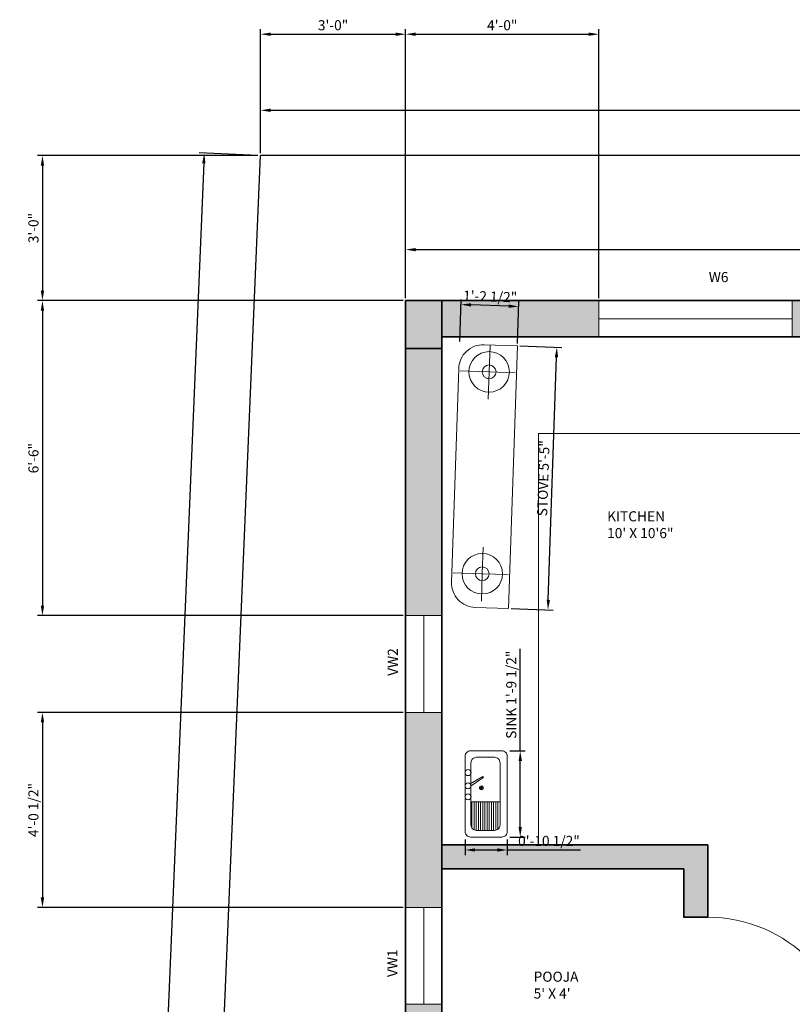
# Model space of a CAD drawing. Units: inches. Extents: x 5395 to 6469, y -203 to 448.
# Tile 3 of 7: x 5395 to 5587, y 204 to 448. Entities that reach past the tile are written whole.
import ezdxf

# ---------------------------------------------------------------- set-up
doc = ezdxf.new("R2010")
doc.units = ezdxf.units.IN
for name, color, linetype, lineweight in [('A-ANNO-DIMS', 2, 'Continuous', 18), ('A-ANNO-TEXT', 6, 'Continuous', 18), ('A-AREA-IDEN', 6, 'Continuous', 18), ('A-COLS', 7, 'Continuous', 35), ('A-COLS-PATT', 2, 'Continuous', 13), ('A-EQPM', 70, 'Continuous', 18), ('A-FLOR-CASE', 32, 'Continuous', 18), ('A-FLOR-FIXT', 70, 'Continuous', 18), ('A-GLAZ', 4, 'Continuous', 18), ('A-WALL', 7, 'Continuous', 35), ('A-WALL-PATT', 11, 'Continuous', 9), ('C-PROP', 7, 'Continuous', 25), ('door', 240, 'Continuous', 18)]:
    doc.layers.add(name, color=color, linetype=linetype, lineweight=lineweight)
doc.styles.get("Standard").update_dxf_attribs({"font": 'arial.ttf'})
doc.dimstyles.new('ISO-25', dxfattribs={"dimtxt": 2.5, "dimasz": 2.5, "dimexe": 1.25, "dimexo": 0.625, "dimtad": 1, "dimdec": 1, "dimlunit": 3, "dimtxsty": 'Standard', "dimcen": 2.5, "dimadec": 0, "dimazin": 0, "dimtfac": 1, "dimtdec": 1, "dimtmove": 0, "dimatfit": 3, "dimfxl": 1, "dimarcsym": 0})

# ---------------------------------------------------------------- blocks, each defined once
blk = doc.blocks.new('*U4')
for p, q in [((0, 0), (0, 5)), ((30, 0), (30, 5))]:
    blk.add_line(p, q)
blk.add_lwpolyline([(0, 0), (0, -30), (1.75, -30), (1.75, 0)], close=True)
blk.add_arc((0, 0), 30, 270, 0)
blk = doc.blocks.new('sink')
for p, q in [((-11.38, 27.19), (-5.63, 30.57)), ((-11.01, 26.26), (-5.62, 29.92)), ((-11.03, 19), (2.23, 19)), ((-10.58, 19), (-10.58, 7)), ((-9.6, 19), (-9.6, 6.16)), ((-8.61, 19), (-8.61, 5.92)), ((-7.63, 19), (-7.63, 5.92)), ((-6.64, 19), (-6.64, 5.92)), ((-5.66, 19), (-5.66, 5.92)), ((-4.67, 19), (-4.67, 5.92)), ((-3.69, 19), (-3.69, 5.92)), ((-2.7, 19), (-2.7, 5.92)), ((-1.72, 19), (-1.72, 5.92)), ((-0.73, 19), (-0.73, 5.92)), ((0.25, 19), (0.25, 5.98)), ((1.23, 19), (1.23, 6.43))]:
    blk.add_line(p, q)
for points in [[(-11.21, 42.26), (3.04, 42.26, -0.414214), (5.54, 39.76), (5.54, 5.38, -0.414214), (3.04, 2.88), (-11.21, 2.88, -0.414214), (-13.71, 5.38), (-13.71, 39.76, -0.414214)], [(-8.53, 39.31), (-0.27, 39.31, -0.414214), (2.23, 36.81), (2.23, 8.42, -0.414214), (-0.27, 5.92), (-8.53, 5.92, -0.414214), (-11.03, 8.42), (-11.03, 36.81, -0.414214)]]:
    blk.add_lwpolyline(points, format="xyb", close=True)
for centre, radius in [((-12.38, 32.33), 1.37), ((-12.38, 26.26), 1.37), ((-12.38, 21.24), 1.37), ((-6.32, 25.41), 0.854), ((-6.32, 25.41), 0.432), ((-6.32, 25.41), 0.203)]:
    blk.add_circle(centre, radius)
blk.add_arc((-5.86, 30.24), 0.398, 306.1138, 55.3114)
blk = doc.blocks.new('STOVE')
for p, q in [((-46.84, 5.62), (-46.82, 11.55)), ((-5.51, 5.62), (-5.49, 11.55)), ((-46.84, 5.62), (-52.42, 5.62)), ((-46.84, 5.62), (-46.84, 0.29)), ((-46.84, 5.62), (-41.4, 5.62)), ((-5.51, 5.62), (-11.1, 5.62)), ((-5.51, 5.62), (-5.51, 0.29)), ((-5.51, 5.62), (-0.08, 5.62))]:
    blk.add_line(p, q)
blk.add_lwpolyline([(-48.78, 11.85), (-5, 11.85, -0.414214), (0, 6.85), (0, 0), (-53.78, 0), (-53.78, 6.85, -0.414214)], format="xyb", close=True)
for centre, radius in [((-46.84, 5.62), 4.14), ((-5.51, 5.62), 4.14), ((-46.84, 5.62), 1.41), ((-5.51, 5.62), 1.41)]:
    blk.add_circle(centre, radius)
blk = doc.blocks.new('*D17')
at = {"layer": 'A-ANNO-DIMS', "color": 0, "lineweight": -2, "transparency": 16777216}
for p, q in [((5490.94, 378.93), (5490.94, 392.2)), ((5493.44, 390.95), (5932.44, 390.95)), ((5934.94, 378.93), (5934.94, 392.2))]:
    blk.add_line(p, q, dxfattribs=at)
at = {"layer": 'A-ANNO-DIMS', "color": 0, "transparency": 16777216}
for points in [[(5493.44, 391.36), (5493.44, 390.53), (5490.94, 390.95)], [(5932.44, 391.36), (5932.44, 390.53), (5934.94, 390.95)]]:
    blk.add_solid(points, dxfattribs=at)
at = {"layer": 'Defpoints', "color": 0, "transparency": 16777216}
for p in [(5934.94, 390.95), (5490.94, 378.31), (5934.94, 378.31)]:
    blk.add_point(p, dxfattribs=at)
at = {"layer": 'A-ANNO-DIMS', "color": 0, "transparency": 16777216, "insert": (5712.94, 393.61), "char_height": 4, "attachment_point": 5}
blk.add_mtext("37'", dxfattribs=at)
blk = doc.blocks.new('*D18')
at = {"layer": 'A-ANNO-DIMS', "color": 0, "lineweight": -2, "transparency": 16777216}
for p, q in [((5454.94, 414.93), (5454.94, 426.78)), ((5457.44, 425.53), (5968.44, 425.53)), ((5970.94, 414.93), (5970.94, 426.78))]:
    blk.add_line(p, q, dxfattribs=at)
at = {"layer": 'A-ANNO-DIMS', "color": 0, "transparency": 16777216}
for points in [[(5457.44, 425.95), (5457.44, 425.12), (5454.94, 425.53)], [(5968.44, 425.95), (5968.44, 425.12), (5970.94, 425.53)]]:
    blk.add_solid(points, dxfattribs=at)
at = {"layer": 'Defpoints', "color": 0, "transparency": 16777216}
for p in [(5970.94, 425.53), (5454.94, 414.31), (5970.94, 414.31)]:
    blk.add_point(p, dxfattribs=at)
at = {"layer": 'A-ANNO-DIMS', "color": 0, "transparency": 16777216, "insert": (5712.94, 428.2), "char_height": 4, "attachment_point": 5}
blk.add_mtext("43'", dxfattribs=at)
blk = doc.blocks.new('*D20')
at = {"layer": 'A-ANNO-DIMS', "color": 0, "lineweight": -2, "transparency": 16777216}
for p, q in [((5454.31, 414.33), (5439.73, 414.95)), ((5440.87, 412.4), (5417.08, -151.61)), ((5430.31, -154.67), (5415.73, -154.05))]:
    blk.add_line(p, q, dxfattribs=at)
at = {"layer": 'A-ANNO-DIMS', "color": 0, "transparency": 16777216}
for points in [[(5440.46, 412.41), (5441.29, 412.38), (5440.98, 414.89)], [(5416.67, -151.59), (5417.5, -151.63), (5416.98, -154.11)]]:
    blk.add_solid(points, dxfattribs=at)
at = {"layer": 'Defpoints', "color": 0, "transparency": 16777216}
for p in [(5454.94, 414.31), (5416.98, -154.11), (5430.94, -154.69)]:
    blk.add_point(p, dxfattribs=at)
at = {"layer": 'A-ANNO-DIMS', "color": 0, "transparency": 16777216, "insert": (5426.32, 130.51), "char_height": 4, "attachment_point": 5, "rotation": 87.5847}
blk.add_mtext('47\'-5.5"', dxfattribs=at)
blk = doc.blocks.new('WINDOW-48IN')
for p, q in [((0, 0), (0, 9)), ((48, 0), (48, 9)), ((0, 4.5), (48, 4.5))]:
    blk.add_line(p, q)
blk = doc.blocks.new('WINDOW-24IN')
for p, q in [((0, 24), (9, 24)), ((4.5, 0), (4.5, 24)), ((0, 0), (9, 0))]:
    blk.add_line(p, q)
blk = doc.blocks.new('*D37')
at = {"layer": 'A-ANNO-DIMS', "color": 0, "lineweight": -2, "transparency": 16777216}
for p, q in [((5519.37, 266.6), (5519.37, 291.93)), ((5516.79, 266.6), (5520.62, 266.6)), ((5519.37, 247.71), (5519.37, 264.1)), ((5516.79, 245.21), (5520.62, 245.21))]:
    blk.add_line(p, q, dxfattribs=at)
at = {"layer": 'A-ANNO-DIMS', "color": 0, "transparency": 16777216}
for points in [[(5518.96, 264.1), (5519.79, 264.1), (5519.37, 266.6)], [(5518.96, 247.71), (5519.79, 247.71), (5519.37, 245.21)]]:
    blk.add_solid(points, dxfattribs=at)
at = {"layer": 'Defpoints', "color": 0, "transparency": 16777216}
for p in [(5516.16, 266.6), (5519.37, 266.6), (5516.16, 245.21)]:
    blk.add_point(p, dxfattribs=at)
at = {"layer": 'A-ANNO-DIMS', "color": 0, "transparency": 16777216, "insert": (5517.46, 280.52), "char_height": 2.5, "attachment_point": 5, "rotation": 90}
blk.add_mtext('SINK 1\'-9 1/2"', dxfattribs=at)
blk = doc.blocks.new('*D38')
at = {"layer": 'A-ANNO-DIMS', "color": 0, "lineweight": -2, "transparency": 16777216}
for p, q in [((5505.69, 244.58), (5505.69, 240.75)), ((5516.16, 244.58), (5516.16, 240.75)), ((5508.19, 242), (5513.66, 242)), ((5516.16, 242), (5534.33, 242))]:
    blk.add_line(p, q, dxfattribs=at)
at = {"layer": 'A-ANNO-DIMS', "color": 0, "transparency": 16777216}
for points in [[(5508.19, 242.41), (5508.19, 241.58), (5505.69, 242)], [(5513.66, 242.41), (5513.66, 241.58), (5516.16, 242)]]:
    blk.add_solid(points, dxfattribs=at)
at = {"layer": 'Defpoints', "color": 0, "transparency": 16777216}
for p in [(5505.69, 245.21), (5516.16, 245.21), (5516.16, 242)]:
    blk.add_point(p, dxfattribs=at)
at = {"layer": 'A-ANNO-DIMS', "color": 0, "transparency": 16777216, "insert": (5526.5, 243.92), "char_height": 2.5, "attachment_point": 5}
blk.add_mtext('0\'-10 1/2"', dxfattribs=at)
blk = doc.blocks.new('*D43')
at = {"layer": 'A-ANNO-DIMS', "color": 0, "lineweight": -2, "transparency": 16777216}
for p, q in [((5519.31, 367.05), (5529.71, 366.69)), ((5526.34, 304.06), (5528.38, 364.24)), ((5517.11, 301.88), (5527.51, 301.52))]:
    blk.add_line(p, q, dxfattribs=at)
at = {"layer": 'A-ANNO-DIMS', "color": 0, "transparency": 16777216}
for points in [[(5527.96, 364.25), (5528.79, 364.22), (5528.46, 366.74)], [(5525.93, 304.08), (5526.76, 304.05), (5526.26, 301.57)]]:
    blk.add_solid(points, dxfattribs=at)
at = {"layer": 'Defpoints', "color": 0, "transparency": 16777216}
for p in [(5518.69, 367.07), (5528.46, 366.74), (5516.48, 301.9)]:
    blk.add_point(p, dxfattribs=at)
at = {"layer": 'A-ANNO-DIMS', "color": 0, "transparency": 16777216, "insert": (5525.44, 334.22), "char_height": 2.5, "attachment_point": 5, "rotation": 88.063}
blk.add_mtext('STOVE 5\'-5"', dxfattribs=at)
blk = doc.blocks.new('*D44')
at = {"layer": 'A-ANNO-DIMS', "color": 0, "lineweight": -2, "transparency": 16777216}
for p, q in [((5504.35, 368.18), (5504.7, 378.58)), ((5516.52, 376.93), (5507.16, 377.24)), ((5518.71, 367.69), (5519.06, 378.09))]:
    blk.add_line(p, q, dxfattribs=at)
at = {"layer": 'A-ANNO-DIMS', "color": 0, "transparency": 16777216}
for points in [[(5507.17, 377.66), (5507.15, 376.83), (5504.66, 377.33)], [(5516.53, 377.34), (5516.5, 376.51), (5519.02, 376.84)]]:
    blk.add_solid(points, dxfattribs=at)
at = {"layer": 'Defpoints', "color": 0, "transparency": 16777216}
for p in [(5504.66, 377.33), (5504.33, 367.55), (5518.69, 367.07)]:
    blk.add_point(p, dxfattribs=at)
at = {"layer": 'A-ANNO-DIMS', "color": 0, "transparency": 16777216, "insert": (5511.9, 379), "char_height": 2.5, "attachment_point": 5, "rotation": 358.063}
blk.add_mtext('1\'-2 1/2"', dxfattribs=at)
blk = doc.blocks.new('*D59')
at = {"layer": 'A-ANNO-DIMS', "color": 0, "lineweight": -2, "transparency": 16777216}
for p, q in [((5454.94, 414.93), (5454.94, 445.66)), ((5490.94, 378.93), (5490.94, 445.66)), ((5457.44, 444.41), (5488.44, 444.41))]:
    blk.add_line(p, q, dxfattribs=at)
at = {"layer": 'A-ANNO-DIMS', "color": 0, "transparency": 16777216}
for points in [[(5457.44, 444.82), (5457.44, 443.99), (5454.94, 444.41)], [(5488.44, 444.82), (5488.44, 443.99), (5490.94, 444.41)]]:
    blk.add_solid(points, dxfattribs=at)
at = {"layer": 'Defpoints', "color": 0, "transparency": 16777216}
for p in [(5490.94, 444.41), (5454.94, 414.31), (5490.94, 378.31)]:
    blk.add_point(p, dxfattribs=at)
at = {"layer": 'A-ANNO-DIMS', "color": 0, "transparency": 16777216, "insert": (5472.94, 446.31), "char_height": 2.5, "attachment_point": 5}
blk.add_mtext('3\'-0"', dxfattribs=at)
blk = doc.blocks.new('*D60')
at = {"layer": 'A-ANNO-DIMS', "color": 0, "lineweight": -2, "transparency": 16777216}
for p, q in [((5454.31, 414.31), (5399.59, 414.31)), ((5400.84, 411.81), (5400.84, 380.81)), ((5490.31, 378.31), (5399.59, 378.31))]:
    blk.add_line(p, q, dxfattribs=at)
at = {"layer": 'A-ANNO-DIMS', "color": 0, "transparency": 16777216}
for points in [[(5400.42, 411.81), (5401.25, 411.81), (5400.84, 414.31)], [(5400.42, 380.81), (5401.25, 380.81), (5400.84, 378.31)]]:
    blk.add_solid(points, dxfattribs=at)
at = {"layer": 'Defpoints', "color": 0, "transparency": 16777216}
for p in [(5454.94, 414.31), (5400.84, 378.31), (5490.94, 378.31)]:
    blk.add_point(p, dxfattribs=at)
at = {"layer": 'A-ANNO-DIMS', "color": 0, "transparency": 16777216, "insert": (5398.93, 396.31), "char_height": 2.5, "attachment_point": 5, "rotation": 90}
blk.add_mtext('3\'-0"', dxfattribs=at)
blk = doc.blocks.new('*D61')
at = {"layer": 'A-ANNO-DIMS', "color": 0, "lineweight": -2, "transparency": 16777216}
for p, q in [((5490.94, 378.93), (5490.94, 445.66)), ((5538.88, 378.93), (5538.88, 445.66)), ((5493.44, 444.41), (5536.38, 444.41))]:
    blk.add_line(p, q, dxfattribs=at)
at = {"layer": 'A-ANNO-DIMS', "color": 0, "transparency": 16777216}
for points in [[(5493.44, 444.82), (5493.44, 443.99), (5490.94, 444.41)], [(5536.38, 444.82), (5536.38, 443.99), (5538.88, 444.41)]]:
    blk.add_solid(points, dxfattribs=at)
at = {"layer": 'Defpoints', "color": 0, "transparency": 16777216}
for p in [(5538.88, 444.41), (5490.94, 378.31), (5538.88, 378.31)]:
    blk.add_point(p, dxfattribs=at)
at = {"layer": 'A-ANNO-DIMS', "color": 0, "transparency": 16777216, "insert": (5514.91, 446.31), "char_height": 2.5, "attachment_point": 5}
blk.add_mtext('4\'-0"', dxfattribs=at)
blk = doc.blocks.new('*D64')
at = {"layer": 'A-ANNO-DIMS', "color": 0, "lineweight": -2, "transparency": 16777216}
for p, q in [((5490.31, 378.31), (5399.59, 378.31)), ((5400.84, 375.81), (5400.84, 302.64)), ((5490.31, 300.14), (5399.59, 300.14))]:
    blk.add_line(p, q, dxfattribs=at)
at = {"layer": 'A-ANNO-DIMS', "color": 0, "transparency": 16777216}
for points in [[(5400.42, 375.81), (5401.25, 375.81), (5400.84, 378.31)], [(5400.42, 302.64), (5401.25, 302.64), (5400.84, 300.14)]]:
    blk.add_solid(points, dxfattribs=at)
at = {"layer": 'Defpoints', "color": 0, "transparency": 16777216}
for p in [(5490.94, 378.31), (5400.84, 300.14), (5490.94, 300.14)]:
    blk.add_point(p, dxfattribs=at)
at = {"layer": 'A-ANNO-DIMS', "color": 0, "transparency": 16777216, "insert": (5398.93, 339.22), "char_height": 2.5, "attachment_point": 5, "rotation": 90}
blk.add_mtext('6\'-6"', dxfattribs=at)
blk = doc.blocks.new('*D65')
at = {"layer": 'A-ANNO-DIMS', "color": 0, "lineweight": -2, "transparency": 16777216}
for p, q in [((5490.31, 276.14), (5399.59, 276.14)), ((5400.84, 273.64), (5400.84, 230.21)), ((5490.31, 227.71), (5399.59, 227.71))]:
    blk.add_line(p, q, dxfattribs=at)
at = {"layer": 'A-ANNO-DIMS', "color": 0, "transparency": 16777216}
for points in [[(5400.42, 273.64), (5401.25, 273.64), (5400.84, 276.14)], [(5400.42, 230.21), (5401.25, 230.21), (5400.84, 227.71)]]:
    blk.add_solid(points, dxfattribs=at)
at = {"layer": 'Defpoints', "color": 0, "transparency": 16777216}
for p in [(5490.94, 276.14), (5400.84, 227.71), (5490.94, 227.71)]:
    blk.add_point(p, dxfattribs=at)
at = {"layer": 'A-ANNO-DIMS', "color": 0, "transparency": 16777216, "insert": (5398.92, 251.92), "char_height": 2.5, "attachment_point": 5, "rotation": 90}
blk.add_mtext('4\'-0 1/2"', dxfattribs=at)

msp = doc.modelspace()

# ---------------------------------------------------------------- hatches: boundary and pattern name
at = {"layer": 'A-COLS-PATT'}
h = msp.add_hatch(color=256, dxfattribs=at)
h.dxf.hatch_style = 1
h.paths.add_polyline_path([(5499.94, 378.31), (5490.94, 378.31), (5490.94, 366.43), (5499.94, 366.43), (5499.94, 369.31)])
at = {"layer": 'A-WALL-PATT'}
h = msp.add_hatch(color=256, dxfattribs=at)
h.dxf.hatch_style = 1
h.paths.add_polyline_path([(5538.88, 378.31), (5499.94, 378.31), (5499.94, 369.31), (5538.88, 369.31)])
h.paths.add_polyline_path([(5499.94, 276.14), (5490.94, 276.14), (5490.94, 227.71), (5499.94, 227.71), (5499.94, 237.31)])
h.paths.add_polyline_path([(5565.94, 243.31), (5499.94, 243.31), (5499.94, 237.31), (5559.94, 237.31), (5559.94, 225.31), (5565.94, 225.31)])
h.paths.add_polyline_path([(5625.94, 367.55), (5619.94, 367.55), (5619.94, 237.31), (5625.94, 237.31)])
h.paths.add_polyline_path([(5745.94, 369.31), (5739.94, 369.31), (5739.94, 237.31), (5745.94, 237.31)])
h.paths.add_polyline_path([(5745.94, 192.25), (5739.94, 192.25), (5739.94, 190.23), (5745.94, 190.23)])
h.paths.add_polyline_path([(5745.94, 180.33), (5739.94, 180.33), (5739.94, 47.04), (5745.94, 47.04)])
h.paths.add_polyline_path([(5877.94, 183.31), (5884.03, 183.31), (5884.03, 189.31), (5747.34, 189.31), (5747.34, 183.31), (5871.94, 183.31), (5871.94, 82.27), (5877.94, 82.27), (5877.94, 90.31), (5925.94, 90.31), (5925.94, 96.31), (5877.94, 96.31)])
h.paths.add_polyline_path([(5934.94, 128.85), (5925.94, 128.85), (5925.94, 55.61), (5934.94, 55.61)])
h.paths.add_polyline_path([(5934.94, 181.4), (5925.94, 181.4), (5925.94, 152.85), (5934.94, 152.85)])
h.paths.add_polyline_path([(5925.94, 189.31), (5914.03, 189.31), (5914.03, 183.31), (5925.94, 183.31)], flags=17)
h.paths.add_polyline_path([(5934.94, 369.31), (5925.94, 369.31), (5925.94, 237.31), (5934.94, 237.31)])
h.paths.add_polyline_path([(5657.93, 378.31), (5627.19, 378.31), (5627.19, 369.31), (5657.93, 369.31)])
h.paths.add_polyline_path([(5619.94, 378.31), (5586.88, 378.31), (5586.88, 369.31), (5619.94, 369.31)])
h.paths.add_polyline_path([(5739.94, 378.31), (5705.93, 378.31), (5705.93, 369.31), (5739.94, 369.31)])
h.paths.add_polyline_path([(5812.1, 378.31), (5753.55, 378.31), (5753.55, 369.31), (5812.1, 369.31)])
h.paths.add_polyline_path([(5923.7, 378.31), (5860.1, 378.31), (5860.1, 369.31), (5923.7, 369.31)])
h.paths.add_polyline_path([(5499.94, 203.71), (5490.94, 203.71), (5490.94, 189.31), (5499.94, 189.31)])
h.paths.add_polyline_path([(5612.93, 189.31), (5499.94, 189.31), (5499.94, 183.31), (5612.93, 183.31)])
h.paths.add_polyline_path([(5499.94, 178.42), (5490.94, 178.42), (5490.94, 132.59), (5499.94, 132.59)])
h.paths.add_polyline_path([(5499.94, 84.59), (5490.94, 84.59), (5490.94, 47.04), (5499.94, 47.04)])
h.paths.add_polyline_path([(5499.94, 11.04), (5490.94, 11.04), (5490.94, 3.31), (5499.94, 3.31)])
h.paths.add_polyline_path([(5532.25, 3.31), (5502.78, 3.31), (5502.78, -5.69), (5532.25, -5.69)])
h.paths.add_polyline_path([(5601.84, 3.31), (5580.25, 3.31), (5580.25, -5.69), (5601.84, -5.69)])
h.paths.add_polyline_path([(5625.94, 3.31), (5614.13, 3.31), (5614.13, -5.69), (5625.94, -5.69)])
h.paths.add_polyline_path([(5787.9, 3.31), (5748.46, 3.31), (5748.46, -5.69), (5787.9, -5.69)])
h.paths.add_polyline_path([(5737.31, 3.31), (5697.94, 3.31), (5697.94, -5.69), (5737.31, -5.69)])
h.paths.add_polyline_path([(5745.94, 11.04), (5739.94, 11.04), (5739.94, 3.31), (5745.94, 3.31)])
h.paths.add_polyline_path([(5922.21, 3.31), (5877.94, 3.31), (5877.94, 46.27), (5871.94, 46.27), (5871.94, 3.31), (5835.9, 3.31), (5835.9, -5.69), (5922.21, -5.69)])
h.paths.add_polyline_path([(5934.94, 31.61), (5925.94, 31.61), (5925.94, 3.31), (5934.94, 3.31)])
h = msp.add_hatch(color=256, dxfattribs=at)
h.dxf.hatch_style = 1
h.paths.add_polyline_path([(5499.94, 366.43), (5490.94, 366.43), (5490.94, 300.14), (5499.94, 300.14)])

# ---------------------------------------------------------------- linework, layer by layer
at = {"layer": 'A-COLS'}
for p, q in [((5499.94, 369.31), (5499.94, 378.31)), ((5499.94, 366.43), (5490.94, 366.43))]:
    msp.add_line(p, q, dxfattribs=at)
at = {"layer": 'A-FLOR-CASE'}
for points in [[(5499.94, 243.31), (5499.94, 369.31), (5619.94, 369.31)], [(5523.94, 243.31), (5523.94, 345.31), (5619.94, 345.31)]]:
    msp.add_lwpolyline(points, dxfattribs=at)
at = {"layer": 'A-WALL'}
for p, q in [((5490.94, 378.31), (5934.94, 378.31)), ((5490.94, 47.04), (5490.94, 378.31)), ((5490.94, 378.31), (5934.94, 378.31)), ((5934.94, 378.31), (5490.94, 378.31)), ((5499.94, 369.31), (5619.94, 369.31)), ((5499.94, 47.04), (5499.94, 369.31)), ((5499.94, 243.31), (5565.94, 243.31)), ((5499.94, 237.31), (5559.94, 237.31))]:
    msp.add_line(p, q, dxfattribs=at)
for points in [[(5565.94, 243.31), (5565.94, 225.31)], [(5499.94, 237.31), (5499.94, 189.31)], [(5559.94, 237.31), (5559.94, 225.31)], [(5559.94, 225.31), (5565.94, 225.31)]]:
    msp.add_lwpolyline(points, dxfattribs=at)
at = {"layer": 'C-PROP'}
for p, q in [((5430.94, -154.69), (5454.94, 414.31)), ((5490.94, 414.31), (5454.94, 414.31)), ((5934.94, 414.31), (5490.94, 414.31))]:
    msp.add_line(p, q, dxfattribs=at)

# ---------------------------------------------------------------- block references
at = {"layer": 'A-EQPM', "xscale": 1.212574967319151, "yscale": 1.212574967319151, "zscale": 1.212574967319151, "rotation": 88.0629585659657}
msp.add_blockref('STOVE', (5518.69, 367.07), dxfattribs=at)
at = {"layer": 'A-FLOR-FIXT', "xscale": 0.5431968377033274, "yscale": 0.5431968377033274, "zscale": 0.5431968377033274}
msp.add_blockref('sink', (5513.15, 243.64), dxfattribs=at)
at = {"layer": 'A-GLAZ'}
for name, p in [('WINDOW-48IN', (5538.88, 369.31)), ('WINDOW-24IN', (5490.94, 276.14)), ('WINDOW-24IN', (5490.94, 203.71))]:
    msp.add_blockref(name, p, dxfattribs=at)
at = {"layer": 'door', "xscale": 1.200014089153335, "yscale": 1.200014089153335, "zscale": 1.200014089153335, "rotation": 90}
msp.add_blockref('*U4', (5565.76, 189.31), dxfattribs=at)

# ---------------------------------------------------------------- texts
at = {"layer": 'A-ANNO-TEXT', "insert": (5566.15, 385.39), "char_height": 2.5, "attachment_point": 1}
msp.add_mtext_dynamic_manual_height_columns('W6', width=62.1492, gutter_width=12.5, heights=[0], dxfattribs=at)
at = {"layer": 'A-ANNO-TEXT', "char_height": 2.5, "attachment_point": 1, "rotation": 90}
for s, insert in [('VW2', (5486.52, 285.21)), ('VW1', (5486.42, 210.47))]:
    msp.add_mtext_dynamic_manual_height_columns(s, width=62.1492, gutter_width=12.5, heights=[0], dxfattribs=dict(at, insert=insert))
at = {"layer": 'A-AREA-IDEN', "char_height": 2.5, "attachment_point": 1}
for s, insert in [('KITCHEN\\P10\' X 10\'6"', (5540.93, 326.04)), ("POOJA\\P5' X 4'", (5522.7, 211.81))]:
    msp.add_mtext_dynamic_manual_height_columns(s, width=62.1492, gutter_width=12.5, heights=[0], dxfattribs=dict(at, insert=insert))

# ---------------------------------------------------------------- dimensions: what is measured, and where the dimension line sits
at = {"layer": 'A-ANNO-DIMS'}
for base, p1, p2, override, picture, middle in [((5490.94, 444.41), (5454.94, 414.31), (5490.94, 378.31), {"dimdec": 1, "dimlfac": 1, "dimrnd": 0, "dimzin": 1, "dimdsep": 46, "dimlunit": 4, "dimfrac": 2}, '*D59', (5472.94, 446.31)), ((5538.88, 444.41), (5490.94, 378.31), (5538.88, 378.31), {"dimdec": 1, "dimlfac": 1, "dimrnd": 0, "dimzin": 1, "dimdsep": 46, "dimlunit": 4, "dimfrac": 2}, '*D61', (5514.91, 446.31)), ((5934.94, 390.95), (5490.94, 378.31), (5934.94, 378.31), {"dimtxt": 4, "dimclrd": 0, "dimclre": 0, "dimclrt": 0}, '*D17', (5712.94, 393.61)), ((5516.16, 242), (5505.69, 245.21), (5516.16, 245.21), {"dimdec": 1, "dimlfac": 1, "dimrnd": 0, "dimzin": 1, "dimdsep": 46, "dimlunit": 4, "dimfrac": 2}, '*D38', (5526.5, 243.92))]:
    dim = msp.add_linear_dim(base=base, p1=p1, p2=p2, dimstyle='ISO-25', override=override, dxfattribs=at)
    dim.commit()
    dim.dimension.update_dxf_attribs({"geometry": picture, "text_midpoint": middle})
for p2, distance, picture, middle in [((5970.94, 414.31), 11.23, '*D18', (5712.94, 428.2)), ((5430.94, -154.69), -13.97, '*D20', (5426.32, 130.51))]:
    dim = msp.add_aligned_dim(p1=(5454.94, 414.31), p2=p2, distance=distance, dimstyle='ISO-25', override={"dimtxt": 4, "dimclrd": 0, "dimclre": 0, "dimclrt": 0}, dxfattribs=at)
    dim.commit()
    dim.dimension.update_dxf_attribs({"geometry": picture, "text_midpoint": middle})
for base, p1, p2, angle, picture, middle in [((5400.84, 378.31), (5454.94, 414.31), (5490.94, 378.31), 90, '*D60', (5398.93, 396.31)), ((5504.66, 377.33), (5518.69, 367.07), (5504.33, 367.55), 178.063, '*D44', (5511.9, 379)), ((5400.84, 300.14), (5490.94, 378.31), (5490.94, 300.14), 90, '*D64', (5398.93, 339.22)), ((5400.84, 227.71), (5490.94, 276.14), (5490.94, 227.71), 90, '*D65', (5398.92, 251.92))]:
    dim = msp.add_linear_dim(base=base, p1=p1, p2=p2, angle=angle, dimstyle='ISO-25', override={"dimdec": 1, "dimlfac": 1, "dimrnd": 0, "dimzin": 1, "dimdsep": 46, "dimlunit": 4, "dimfrac": 2}, dxfattribs=at)
    dim.commit()
    dim.dimension.update_dxf_attribs({"geometry": picture, "text_midpoint": middle})
for base, p1, p2, angle, text, picture, middle in [((5528.46, 366.74), (5516.48, 301.9), (5518.69, 367.07), 88.063, 'STOVE <>', '*D43', (5525.44, 334.22)), ((5519.37, 266.6), (5516.16, 245.21), (5516.16, 266.6), 90, 'SINK <>', '*D37', (5517.46, 280.52))]:
    dim = msp.add_linear_dim(base=base, p1=p1, p2=p2, angle=angle, text=text, dimstyle='ISO-25', override={"dimdec": 1, "dimlfac": 1, "dimrnd": 0, "dimzin": 1, "dimdsep": 46, "dimlunit": 4, "dimfrac": 2}, dxfattribs=at)
    dim.commit()
    dim.dimension.update_dxf_attribs({"geometry": picture, "text_midpoint": middle})

doc.saveas('drawing.dxf')
